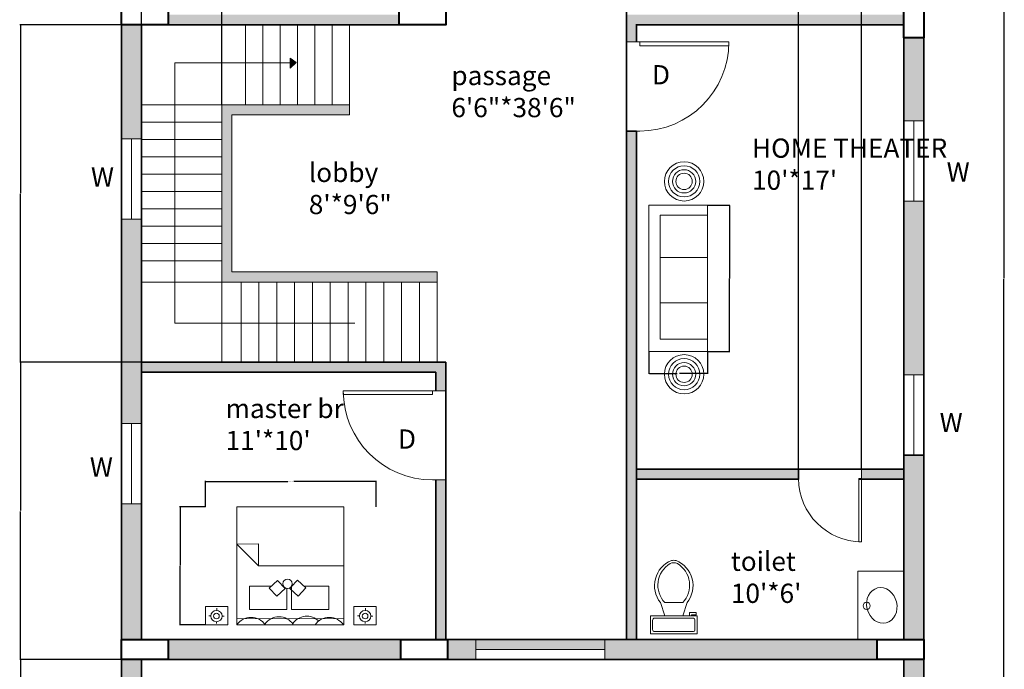
# Model space of a CAD drawing. Units: inches. Extents: x 1568 to 2529, y 2149 to 2897.
# Tile 15 of 16: x 2087 to 2529, y 2326 to 2618. Entities that reach past the tile are written whole.
import ezdxf

# ---------------------------------------------------------------- set-up
doc = ezdxf.new("R2010")
doc.units = ezdxf.units.IN
for name, color, linetype, lineweight in [('A-ANNO-DIMS', 2, 'Continuous', 18), ('A-ANNO-SYMB', 7, 'Continuous', 18), ('A-AREA-IDEN', 210, 'Continuous', 18), ('A-COLS', 7, 'Continuous', 40), ('A-DOOR', 4, 'Continuous', 18), ('A-EQPM', 8, 'Continuous', 18), ('A-FLOR-FIXT', 9, 'Continuous', 18), ('A-FLOR-STRS', 7, 'Continuous', 18), ('A-FURN', 8, 'Continuous', 18), ('A-WALL-PATT', 172, 'Continuous', 13), ('text', 210, 'Continuous', 18), ('wall', 7, 'Continuous', 35), ('window', 130, 'Continuous', 18)]:
    doc.layers.add(name, color=color, linetype=linetype, lineweight=lineweight)
doc.styles.get("Standard").update_dxf_attribs({"font": 'arial.ttf'})
doc.dimstyles.get("Standard").update_dxf_attribs({"dimtxt": 0.18, "dimasz": 0.18, "dimexe": 0.18, "dimexo": 0.0625, "dimgap": 0.09, "dimtad": 0, "dimtih": 1, "dimtoh": 1, "dimdec": 4, "dimzin": 0, "dimdsep": 46, "dimtxsty": 'Standard', "dimcen": 0.09, "dimadec": 0, "dimazin": 0, "dimtfac": 1, "dimtdec": 4, "dimtofl": 0, "dimtmove": 0, "dimatfit": 3, "dimfxl": 1, "dimtolj": 1, "dimtzin": 0, "dimarcsym": 0})

# ---------------------------------------------------------------- blocks, each defined once
blk = doc.blocks.new('*U2')
for p, q in [((0, 0), (0, -6)), ((40, 0), (40, -6))]:
    blk.add_line(p, q)
blk.add_lwpolyline([(0, 0), (0, 40), (1.75, 40), (1.75, 0)], close=True)
blk.add_arc((0, 0), 40, 0, 90)
blk = doc.blocks.new('*U4')
for p, q in [((9.5, -6), (9.5, -2)), ((-10, -8.5), (-8, -8.5)), ((-10, -9.5), (-10, -8.5)), ((-8, -8.5), (-8, -8)), ((-7, -8), (-7, -9.5)), ((-4, -8), (-6, -14)), ((4, -8), (6, -14)), ((-7, -9.5), (-10, -9.5)), ((4, -14), (-4, -14))]:
    blk.add_line(p, q)
blk.add_lwpolyline([(10.5, -8), (10.5, 0), (-10.5, 0), (-10.5, -8)], close=True)
for points in [[(-9.5, -2), (-9.5, -6)], [(8.5, -1), (-8.5, -1)], [(-8.5, -7), (8.5, -7)]]:
    blk.add_lwpolyline(points)
for centre, radius, start, end in [((-8.62, -1.88), 0.884, 81.8699, 188.1301), ((8.62, -1.88), 0.884, 351.8699, 98.1301), ((-8.62, -6.12), 0.884, 171.8699, 278.1301), ((8.62, -6.12), 0.884, 261.8699, 8.1301), ((3.52, -21.58), 12.17, 141.4691, 247.9714), ((4.2, -21.82), 11.33, 136.3677, 238.9468), ((-3.52, -21.58), 12.17, 292.0284, 38.5307), ((-4.2, -21.82), 11.33, 301.053, 43.6321), ((0, -27.88), 4, 245.7318, 294.2682), ((0, -29), 4, 254.8605, 285.1395)]:
    blk.add_arc(centre, radius, start, end)
blk = doc.blocks.new('BED-WITH-NIGHTSTANDS')
for p, q in [((14.05, 36.12), (23.68, 36.4)), ((23.68, 26.45), (14.05, 36.12)), ((23.68, 36.4), (23.68, 26.45)), ((61.95, 26.45), (23.68, 26.45)), ((38.01, 16.14), (37.63, 16.49)), ((38.35, 15.84), (38.01, 16.14)), ((38.35, 16.98), (38.35, 15.84)), ((5, 6.48), (5, 7.42)), ((71.71, 6.48), (71.71, 7.42)), ((2.29, 3.95), (1.38, 3.95)), ((4.92, 1.35), (4.92, 0.55)), ((7.42, 3.92), (8.29, 3.92)), ((14.05, 2.79), (61.95, 2.73)), ((69, 3.95), (68.1, 3.95)), ((71.64, 1.35), (71.64, 0.55)), ((74.13, 3.92), (75, 3.92))]:
    blk.add_line(p, q)
for points in [[(14.05, 0), (61.95, 0), (61.95, 52.9), (14.05, 52.9)], [(31.9, 12.77), (35.7, 16.21), (32.32, 19.94), (28.52, 16.5)], [(10.04, 0), (0, 0), (0, 8.21), (10.04, 8.21)], [(76.49, 0), (66.44, 0), (66.44, 8.21), (76.49, 8.21)]]:
    blk.add_lwpolyline(points, close=True)
for points in [[(38.35, 16.98), (41.16, 20.08), (44.96, 16.64), (41.58, 12.91), (38.01, 16.14)], [(29.36, 17.26), (19.65, 17.26), (19.65, 6.93), (36.45, 6.93), (36.45, 16.34)], [(35.04, 17.26), (34.75, 17.26)], [(38.52, 17.23), (38.52, 6.93), (55.32, 6.93), (55.32, 17.26), (44.28, 17.26)], [(38.6, 17.26), (38.54, 17.26)]]:
    blk.add_lwpolyline(points)
for centre, radius in [((36.79, 18.4), 2.09), ((4.85, 3.92), 2.56), ((4.85, 3.92), 1.27), ((71.57, 3.92), 2.56), ((71.57, 3.92), 1.27)]:
    blk.add_circle(centre, radius)
for centre, start in [((20.4, -4.37), 34.5304), ((32.9, -4.09), 34.5304), ((45.42, -3.86), 46.3255), ((55.47, -4.37), 34.5304)]:
    blk.add_arc(centre, 7.71, start, 145.4696)
blk = doc.blocks.new('SOFA-THREE-SEAT')
for p, q in [((0, 60.18), (0, 65.7)), ((0, 65.7), (26.25, 65.7)), ((26.25, 65.7), (26.25, 0)), ((0, 43.78), (21.18, 43.78)), ((0, 23.43), (21.18, 23.43)), ((0, 0), (0, 5.84)), ((26.25, 0), (0, 0))]:
    blk.add_line(p, q)
blk.add_lwpolyline([(21.18, 60.18), (0, 60.18), (0, 4.48), (21.18, 4.48)], close=True)
blk = doc.blocks.new('TABLE-ROUND-END')
for radius in [8.82, 7, 5.22, 3.67]:
    blk.add_circle((0, 0), radius)
blk = doc.blocks.new('*D17')
at = {"layer": 'A-ANNO-DIMS', "color": 0, "lineweight": -2, "transparency": 16777216}
for p, q in [((2170.58, 2399.15), (2170.58, 2410.74)), ((2170.76, 2410.56), (2207.51, 2410.56)), ((2246.88, 2410.56), (2210.13, 2410.56)), ((2247.06, 2399.15), (2247.06, 2410.74))]:
    blk.add_line(p, q, dxfattribs=at)
at = {"layer": 'A-ANNO-DIMS', "color": 0, "transparency": 16777216}
for points in [[(2170.76, 2410.59), (2170.76, 2410.53), (2170.58, 2410.56)], [(2246.88, 2410.59), (2246.88, 2410.53), (2247.06, 2410.56)]]:
    blk.add_solid(points, dxfattribs=at)
at = {"layer": 'Defpoints', "color": 0, "transparency": 16777216}
for p in [(2247.06, 2410.56), (2170.58, 2399.09), (2247.06, 2399.09)]:
    blk.add_point(p, dxfattribs=at)
at = {"layer": 'A-ANNO-DIMS', "color": 0, "transparency": 16777216, "insert": (2208.82, 2410.56), "char_height": 0.18, "attachment_point": 5}
blk.add_mtext('\\A1;BED GROUP 76 TYP.', dxfattribs=at)
blk = doc.blocks.new('*D18')
at = {"layer": 'A-ANNO-DIMS', "color": 0, "lineweight": -2, "transparency": 16777216}
for p, q in [((2170.51, 2399.09), (2158.92, 2399.09)), ((2159.1, 2398.91), (2159.1, 2372.82)), ((2159.1, 2346.37), (2159.1, 2372.46)), ((2170.51, 2346.19), (2158.92, 2346.19))]:
    blk.add_line(p, q, dxfattribs=at)
at = {"layer": 'A-ANNO-DIMS', "color": 0, "transparency": 16777216}
for points in [[(2159.07, 2398.91), (2159.13, 2398.91), (2159.1, 2399.09)], [(2159.07, 2346.37), (2159.13, 2346.37), (2159.1, 2346.19)]]:
    blk.add_solid(points, dxfattribs=at)
at = {"layer": 'Defpoints', "color": 0, "transparency": 16777216}
for p in [(2159.1, 2399.09), (2170.58, 2399.09), (2170.58, 2346.19)]:
    blk.add_point(p, dxfattribs=at)
at = {"layer": 'A-ANNO-DIMS', "color": 0, "transparency": 16777216, "insert": (2159.1, 2372.64), "char_height": 0.18, "attachment_point": 5}
blk.add_mtext('\\A1;53 TYP.', dxfattribs=at)
blk = doc.blocks.new('*D21')
at = {"layer": 'A-ANNO-DIMS', "color": 0, "lineweight": -2, "transparency": 16777216}
for p, q in [((2395.82, 2534.49), (2405.79, 2534.49)), ((2405.61, 2534.31), (2405.61, 2501.83)), ((2405.61, 2468.98), (2405.61, 2501.46)), ((2395.82, 2468.8), (2405.79, 2468.8))]:
    blk.add_line(p, q, dxfattribs=at)
at = {"layer": 'A-ANNO-DIMS', "color": 0, "transparency": 16777216}
for points in [[(2405.58, 2534.31), (2405.64, 2534.31), (2405.61, 2534.49)], [(2405.58, 2468.98), (2405.64, 2468.98), (2405.61, 2468.8)]]:
    blk.add_solid(points, dxfattribs=at)
at = {"layer": 'Defpoints', "color": 0, "transparency": 16777216}
for p in [(2395.75, 2534.49), (2395.75, 2468.8), (2405.61, 2468.8)]:
    blk.add_point(p, dxfattribs=at)
at = {"layer": 'A-ANNO-DIMS', "color": 0, "transparency": 16777216, "insert": (2405.61, 2501.65), "char_height": 0.18, "attachment_point": 5}
blk.add_mtext('\\A1;SOFA 66 TYP.', dxfattribs=at)
blk = doc.blocks.new('*D22')
at = {"layer": 'A-ANNO-DIMS', "color": 0, "lineweight": -2, "transparency": 16777216}
for p, q in [((2369.51, 2468.74), (2369.51, 2458.76)), ((2395.75, 2468.74), (2395.75, 2458.76)), ((2369.69, 2458.94), (2382.1, 2458.94)), ((2395.57, 2458.94), (2383.16, 2458.94))]:
    blk.add_line(p, q, dxfattribs=at)
at = {"layer": 'A-ANNO-DIMS', "color": 0, "transparency": 16777216}
for points in [[(2369.69, 2458.97), (2369.69, 2458.91), (2369.51, 2458.94)], [(2395.57, 2458.97), (2395.57, 2458.91), (2395.75, 2458.94)]]:
    blk.add_solid(points, dxfattribs=at)
at = {"layer": 'Defpoints', "color": 0, "transparency": 16777216}
for p in [(2369.51, 2468.8), (2395.75, 2468.8), (2369.51, 2458.94)]:
    blk.add_point(p, dxfattribs=at)
at = {"layer": 'A-ANNO-DIMS', "color": 0, "transparency": 16777216, "insert": (2382.63, 2458.94), "char_height": 0.18, "attachment_point": 5}
blk.add_mtext('\\A1;26 TYP.', dxfattribs=at)
blk = doc.blocks.new('*D38')
at = {"layer": 'A-ANNO-DIMS', "color": 0, "lineweight": -2, "transparency": 16777216}
for p, q in [((2492.94, 2801.53), (2528.91, 2801.53)), ((2528.73, 2801.35), (2528.73, 2501.71)), ((2528.73, 2201.71), (2528.73, 2501.35)), ((2492.91, 2201.53), (2528.91, 2201.53))]:
    blk.add_line(p, q, dxfattribs=at)
at = {"layer": 'A-ANNO-DIMS', "color": 0, "transparency": 16777216}
for points in [[(2528.7, 2801.35), (2528.76, 2801.35), (2528.73, 2801.53)], [(2528.7, 2201.71), (2528.76, 2201.71), (2528.73, 2201.53)]]:
    blk.add_solid(points, dxfattribs=at)
at = {"layer": 'Defpoints', "color": 0, "transparency": 16777216}
for p in [(2492.88, 2801.53), (2528.73, 2801.53), (2492.85, 2201.53)]:
    blk.add_point(p, dxfattribs=at)
at = {"layer": 'A-ANNO-DIMS', "color": 0, "transparency": 16777216, "insert": (2528.73, 2501.53), "char_height": 0.18, "attachment_point": 5}
blk.add_mtext('\\A1;600', dxfattribs=at)
blk = doc.blocks.new('*D39')
at = {"layer": 'A-ANNO-DIMS', "color": 0, "lineweight": -2, "transparency": 16777216}
for p, q in [((2132.79, 2330.53), (2087.29, 2330.53)), ((2087.47, 2330.35), (2087.47, 2266.21)), ((2087.47, 2201.71), (2087.47, 2265.85)), ((2132.79, 2201.53), (2087.29, 2201.53))]:
    blk.add_line(p, q, dxfattribs=at)
at = {"layer": 'A-ANNO-DIMS', "color": 0, "transparency": 16777216}
for points in [[(2087.44, 2330.35), (2087.5, 2330.35), (2087.47, 2330.53)], [(2087.44, 2201.71), (2087.5, 2201.71), (2087.47, 2201.53)]]:
    blk.add_solid(points, dxfattribs=at)
at = {"layer": 'Defpoints', "color": 0, "transparency": 16777216}
for p in [(2087.47, 2330.53), (2132.85, 2330.53), (2132.85, 2201.53)]:
    blk.add_point(p, dxfattribs=at)
at = {"layer": 'A-ANNO-DIMS', "color": 0, "transparency": 16777216, "insert": (2087.47, 2266.03), "char_height": 0.18, "attachment_point": 5}
blk.add_mtext('\\A1;129', dxfattribs=at)
blk = doc.blocks.new('*D40')
at = {"layer": 'A-ANNO-DIMS', "color": 0, "lineweight": -2, "transparency": 16777216}
for p, q in [((2141.79, 2464.03), (2087.29, 2464.03)), ((2087.47, 2463.85), (2087.47, 2397.46)), ((2087.47, 2330.71), (2087.47, 2397.1)), ((2141.79, 2330.53), (2087.29, 2330.53))]:
    blk.add_line(p, q, dxfattribs=at)
at = {"layer": 'A-ANNO-DIMS', "color": 0, "transparency": 16777216}
for points in [[(2087.44, 2463.85), (2087.5, 2463.85), (2087.47, 2464.03)], [(2087.44, 2330.71), (2087.5, 2330.71), (2087.47, 2330.53)]]:
    blk.add_solid(points, dxfattribs=at)
at = {"layer": 'Defpoints', "color": 0, "transparency": 16777216}
for p in [(2087.47, 2464.03), (2141.85, 2464.03), (2141.85, 2330.53)]:
    blk.add_point(p, dxfattribs=at)
at = {"layer": 'A-ANNO-DIMS', "color": 0, "transparency": 16777216, "insert": (2087.47, 2397.28), "char_height": 0.18, "attachment_point": 5}
blk.add_mtext('\\A1;133.5', dxfattribs=at)
blk = doc.blocks.new('*D41')
at = {"layer": 'A-ANNO-DIMS', "color": 0, "lineweight": -2, "transparency": 16777216}
for p, q in [((2141.79, 2615.53), (2087.29, 2615.53)), ((2087.47, 2615.35), (2087.47, 2539.96)), ((2087.47, 2464.21), (2087.47, 2539.6)), ((2141.79, 2464.03), (2087.29, 2464.03))]:
    blk.add_line(p, q, dxfattribs=at)
at = {"layer": 'A-ANNO-DIMS', "color": 0, "transparency": 16777216}
for points in [[(2087.44, 2615.35), (2087.5, 2615.35), (2087.47, 2615.53)], [(2087.44, 2464.21), (2087.5, 2464.21), (2087.47, 2464.03)]]:
    blk.add_solid(points, dxfattribs=at)
at = {"layer": 'Defpoints', "color": 0, "transparency": 16777216}
for p in [(2087.47, 2615.53), (2141.85, 2615.53), (2141.85, 2464.03)]:
    blk.add_point(p, dxfattribs=at)
at = {"layer": 'A-ANNO-DIMS', "color": 0, "transparency": 16777216, "insert": (2087.47, 2539.78), "char_height": 0.18, "attachment_point": 5}
blk.add_mtext('\\A1;151.5', dxfattribs=at)
blk = doc.blocks.new('*D42')
at = {"layer": 'A-ANNO-DIMS', "color": 0, "lineweight": -2, "transparency": 16777216}
for p, q in [((2141.85, 2579.59), (2141.85, 2896.84)), ((2142.03, 2896.66), (2159.63, 2896.66)), ((2177.67, 2896.66), (2160.07, 2896.66)), ((2177.85, 2579.59), (2177.85, 2896.84))]:
    blk.add_line(p, q, dxfattribs=at)
at = {"layer": 'A-ANNO-DIMS', "color": 0, "transparency": 16777216}
for points in [[(2142.03, 2896.69), (2142.03, 2896.63), (2141.85, 2896.66)], [(2177.67, 2896.69), (2177.67, 2896.63), (2177.85, 2896.66)]]:
    blk.add_solid(points, dxfattribs=at)
at = {"layer": 'Defpoints', "color": 0, "transparency": 16777216}
for p in [(2177.85, 2896.66), (2141.85, 2579.53), (2177.85, 2579.53)]:
    blk.add_point(p, dxfattribs=at)
at = {"layer": 'A-ANNO-DIMS', "color": 0, "transparency": 16777216, "insert": (2159.85, 2896.66), "char_height": 0.18, "attachment_point": 5}
blk.add_mtext('\\A1;36', dxfattribs=at)
blk = doc.blocks.new('*D45')
at = {"layer": 'A-ANNO-DIMS', "color": 0, "lineweight": -2, "transparency": 16777216}
for p, q in [((2436.62, 2416.09), (2436.62, 2896.84)), ((2436.8, 2896.66), (2450.31, 2896.66)), ((2464.75, 2896.66), (2451.24, 2896.66)), ((2464.93, 2416.09), (2464.93, 2896.84))]:
    blk.add_line(p, q, dxfattribs=at)
at = {"layer": 'A-ANNO-DIMS', "color": 0, "transparency": 16777216}
for points in [[(2436.8, 2896.69), (2436.8, 2896.63), (2436.62, 2896.66)], [(2464.75, 2896.69), (2464.75, 2896.63), (2464.93, 2896.66)]]:
    blk.add_solid(points, dxfattribs=at)
at = {"layer": 'Defpoints', "color": 0, "transparency": 16777216}
for p in [(2464.93, 2896.66), (2436.62, 2416.03), (2464.93, 2416.03)]:
    blk.add_point(p, dxfattribs=at)
at = {"layer": 'A-ANNO-DIMS', "color": 0, "transparency": 16777216, "insert": (2450.77, 2896.66), "char_height": 0.18, "attachment_point": 5}
blk.add_mtext('\\A1;28.305', dxfattribs=at)

msp = doc.modelspace()

# ---------------------------------------------------------------- hatches: boundary and pattern name
at = {"layer": 'A-ANNO-SYMB'}
h = msp.add_hatch(color=256, dxfattribs=at)
h.dxf.hatch_style = 1
h.paths.add_polyline_path([(2211.1402, 2598.4963), (2208.5798, 2600.5832), (2208.5798, 2596.9578), (2208.5798, 2595.9578)])
at = {"layer": 'A-WALL-PATT'}
h = msp.add_hatch(color=256, dxfattribs=at)
h.dxf.hatch_style = 1
h.paths.add_polyline_path([(2257.4593, 2801.532), (2153.7841, 2801.532), (2153.7841, 2792.532), (2257.4593, 2792.532)])
h.paths.add_polyline_path([(2331.7115, 2801.532), (2278.3925, 2801.532), (2278.3925, 2792.532), (2331.7115, 2792.532)])
h.paths.add_polyline_path([(2141.8509, 2753.3576), (2141.6865, 2753.3576), (2132.8509, 2753.3576), (2132.8509, 2705.9172), (2141.8509, 2705.9172)])
h.paths.add_polyline_path([(2278.3509, 2757.9833), (2274.1052, 2757.9833, -0.00224577), (2273.8509, 2757.9844), (2273.8509, 2744.532), (2141.8509, 2744.532), (2141.8509, 2740.032), (2273.8509, 2740.032), (2273.8509, 2730.8156), (2278.3509, 2730.8156), (2278.3509, 2740.032)])
h.paths.add_polyline_path([(2471.947, 2801.532), (2367.7115, 2801.532), (2367.7115, 2792.532), (2471.947, 2792.532)])
h.paths.add_polyline_path([(2402.7886, 2351.2573), (2436.5067, 2351.2573), (2436.5067, 2383.453), (2402.7886, 2383.453)], flags=9)
h.paths.add_polyline_path([(2363.115, 2703.2844), (2384.1733, 2703.2844), (2384.1733, 2721.0645), (2363.115, 2721.0645)], flags=9)
h.paths.add_polyline_path([(2367.7631, 2584.032), (2380.7818, 2584.032), (2380.7818, 2601.8121), (2367.7631, 2601.8121)], flags=9)
h.paths.add_polyline_path([(2412.2706, 2522.1491), (2473.8683, 2522.1491), (2473.8683, 2568.725), (2412.2706, 2568.725)], flags=9)
h.paths.add_polyline_path([(2412.2706, 2686.5293), (2474.6569, 2686.5293), (2474.6569, 2718.725), (2412.2706, 2718.725)], flags=9)
h.paths.add_polyline_path([(2305.8704, 2205.7429), (2329.6007, 2205.7429), (2329.6007, 2223.523), (2305.8704, 2223.523)], flags=9)
h.paths.add_polyline_path([(2312.4696, 2308.5242), (2328.1604, 2308.5242), (2328.1604, 2326.3043), (2312.4696, 2326.3043)], flags=9)
h.paths.add_polyline_path([(2253.7912, 2420.5203), (2266.8099, 2420.5203), (2266.8099, 2438.3004), (2253.7912, 2438.3004)], flags=9)
h.paths.add_polyline_path([(2261.5714, 2703.4315), (2274.5902, 2703.4315), (2274.5902, 2721.2116), (2261.5714, 2721.2116)], flags=9)
h.paths.add_polyline_path([(2277.898, 2569.2764), (2333.9221, 2569.2764), (2333.9221, 2601.4721), (2277.898, 2601.4721)], flags=9)
h.paths.add_polyline_path([(2176.0749, 2419.8331), (2231.9754, 2419.8331), (2231.9754, 2452.0288), (2176.0749, 2452.0288)], flags=9)
h.paths.add_polyline_path([(2213.9423, 2525.7697), (2252.2216, 2525.7697), (2252.2216, 2557.9653), (2213.9423, 2557.9653)], flags=9)
h.paths.add_polyline_path([(2170.6878, 2692.4783), (2211.1801, 2692.4783), (2211.1801, 2724.6739), (2170.6878, 2724.6739)], flags=9)
h.paths.add_polyline_path([(2262.4629, 2764.5694), (2275.4816, 2764.5694), (2275.4816, 2782.3495), (2262.4629, 2782.3495)], flags=9)
h.paths.add_polyline_path([(2183.6493, 2749.7187), (2217.3673, 2749.7187), (2217.3673, 2781.9143), (2183.6493, 2781.9143)], flags=9)
h = msp.add_hatch(color=256, dxfattribs=at)
h.dxf.hatch_style = 1
h.paths.add_polyline_path([(2492.8509, 2792.532), (2483.8509, 2792.532), (2483.8509, 2699.1671), (2492.8509, 2699.1671)])
h.paths.add_polyline_path([(2278.3509, 2690.8156), (2273.8509, 2690.8156), (2273.8509, 2624.532), (2278.3509, 2624.532)])
h.paths.add_polyline_path([(2257.4177, 2620.032), (2153.7841, 2620.032), (2153.7841, 2615.532), (2257.4177, 2615.532)])
h.paths.add_polyline_path([(2141.8509, 2669.9172), (2132.8509, 2669.9172), (2132.8509, 2624.532), (2141.8509, 2624.532)])
h.paths.add_polyline_path([(2402.7886, 2351.2573), (2436.5067, 2351.2573), (2436.5067, 2383.453), (2402.7886, 2383.453)], flags=9)
h.paths.add_polyline_path([(2363.115, 2703.2844), (2384.1733, 2703.2844), (2384.1733, 2721.0645), (2363.115, 2721.0645)], flags=9)
h.paths.add_polyline_path([(2367.7631, 2584.032), (2380.7818, 2584.032), (2380.7818, 2601.8121), (2367.7631, 2601.8121)], flags=9)
h.paths.add_polyline_path([(2412.2706, 2522.1491), (2473.8683, 2522.1491), (2473.8683, 2568.725), (2412.2706, 2568.725)], flags=9)
h.paths.add_polyline_path([(2412.2706, 2686.5293), (2474.6569, 2686.5293), (2474.6569, 2718.725), (2412.2706, 2718.725)], flags=9)
h.paths.add_polyline_path([(2305.8704, 2205.7429), (2329.6007, 2205.7429), (2329.6007, 2223.523), (2305.8704, 2223.523)], flags=9)
h.paths.add_polyline_path([(2312.4696, 2308.5242), (2328.1604, 2308.5242), (2328.1604, 2326.3043), (2312.4696, 2326.3043)], flags=9)
h.paths.add_polyline_path([(2253.7912, 2420.5203), (2266.8099, 2420.5203), (2266.8099, 2438.3004), (2253.7912, 2438.3004)], flags=9)
h.paths.add_polyline_path([(2261.5714, 2703.4315), (2274.5902, 2703.4315), (2274.5902, 2721.2116), (2261.5714, 2721.2116)], flags=9)
h.paths.add_polyline_path([(2262.4629, 2764.5694), (2275.4816, 2764.5694), (2275.4816, 2782.3495), (2262.4629, 2782.3495)], flags=9)
h.paths.add_polyline_path([(2277.898, 2569.2764), (2333.9221, 2569.2764), (2333.9221, 2601.4721), (2277.898, 2601.4721)], flags=9)
h.paths.add_polyline_path([(2176.0749, 2419.8331), (2231.9754, 2419.8331), (2231.9754, 2452.0288), (2176.0749, 2452.0288)], flags=9)
h.paths.add_polyline_path([(2213.9423, 2525.7697), (2252.2216, 2525.7697), (2252.2216, 2557.9653), (2213.9423, 2557.9653)], flags=9)
h.paths.add_polyline_path([(2170.6878, 2692.4783), (2211.1801, 2692.4783), (2211.1801, 2724.6739), (2170.6878, 2724.6739)], flags=9)
h.paths.add_polyline_path([(2183.6493, 2749.7187), (2217.3673, 2749.7187), (2217.3673, 2781.9143), (2183.6493, 2781.9143)], flags=9)
h = msp.add_hatch(color=256, dxfattribs=at)
h.dxf.hatch_style = 1
h.paths.add_polyline_path([(2141.8509, 2615.532), (2132.8509, 2615.532), (2132.8509, 2564.2764), (2141.8509, 2564.2764)])
h.paths.add_polyline_path([(2141.8509, 2528.2764), (2132.8509, 2528.2764), (2132.8509, 2436.512), (2141.8509, 2436.512), (2141.8509, 2459.532)])
h.paths.add_polyline_path([(2278.3509, 2464.032), (2253.6925, 2464.032), (2141.8509, 2464.032), (2141.8509, 2459.532), (2255.8509, 2459.532), (2273.8509, 2459.532), (2273.8509, 2451.2271), (2278.3509, 2451.2271)])
h.paths.add_polyline_path([(2141.8509, 2400.512), (2132.8509, 2400.512), (2132.8509, 2339.532), (2141.8509, 2339.532)])
h.paths.add_polyline_path([(2258.2144, 2339.532), (2153.7841, 2339.532), (2153.7841, 2330.532), (2258.2144, 2330.532)])
h.paths.add_polyline_path([(2291.8353, 2339.532), (2279.1476, 2339.532), (2279.1476, 2330.532), (2291.8353, 2330.532)])
h.paths.add_polyline_path([(2402.7886, 2351.2573), (2436.5067, 2351.2573), (2436.5067, 2383.453), (2402.7886, 2383.453)], flags=9)
h.paths.add_polyline_path([(2363.115, 2703.2844), (2384.1733, 2703.2844), (2384.1733, 2721.0645), (2363.115, 2721.0645)], flags=9)
h.paths.add_polyline_path([(2367.7631, 2584.032), (2380.7818, 2584.032), (2380.7818, 2601.8121), (2367.7631, 2601.8121)], flags=9)
h.paths.add_polyline_path([(2412.2706, 2522.1491), (2473.8683, 2522.1491), (2473.8683, 2568.725), (2412.2706, 2568.725)], flags=9)
h.paths.add_polyline_path([(2412.2706, 2686.5293), (2474.6569, 2686.5293), (2474.6569, 2718.725), (2412.2706, 2718.725)], flags=9)
h.paths.add_polyline_path([(2305.8704, 2205.7429), (2329.6007, 2205.7429), (2329.6007, 2223.523), (2305.8704, 2223.523)], flags=9)
h.paths.add_polyline_path([(2312.4696, 2308.5242), (2328.1604, 2308.5242), (2328.1604, 2326.3043), (2312.4696, 2326.3043)], flags=9)
h.paths.add_polyline_path([(2261.5714, 2703.4315), (2274.5902, 2703.4315), (2274.5902, 2721.2116), (2261.5714, 2721.2116)], flags=9)
h.paths.add_polyline_path([(2262.4629, 2764.5694), (2275.4816, 2764.5694), (2275.4816, 2782.3495), (2262.4629, 2782.3495)], flags=9)
h.paths.add_polyline_path([(2277.898, 2569.2764), (2333.9221, 2569.2764), (2333.9221, 2601.4721), (2277.898, 2601.4721)], flags=9)
h.paths.add_polyline_path([(2213.9423, 2525.7697), (2252.2216, 2525.7697), (2252.2216, 2557.9653), (2213.9423, 2557.9653)], flags=9)
h.paths.add_polyline_path([(2170.6878, 2692.4783), (2211.1801, 2692.4783), (2211.1801, 2724.6739), (2170.6878, 2724.6739)], flags=9)
h.paths.add_polyline_path([(2183.6493, 2749.7187), (2217.3673, 2749.7187), (2217.3673, 2781.9143), (2183.6493, 2781.9143)], flags=9)
h = msp.add_hatch(color=256, dxfattribs=at)
h.dxf.hatch_style = 1
h.paths.add_polyline_path([(2492.8509, 2663.1671), (2483.8509, 2663.1671), (2483.8509, 2630.5978), (2492.8509, 2630.5978)])
h.paths.add_polyline_path([(2492.8509, 2609.6646), (2483.8509, 2609.6646), (2483.8509, 2572.3679), (2492.8509, 2572.3679)])
h.paths.add_polyline_path([(2492.8509, 2536.3679), (2483.8509, 2536.3679), (2483.8509, 2476.032), (2483.8509, 2458.371), (2492.8509, 2458.371)])
h.paths.add_polyline_path([(2483.8509, 2620.032), (2361.425, 2620.032), (2359.3509, 2620.032), (2359.3509, 2607.8035), (2363.8509, 2607.8035), (2363.8509, 2615.532), (2483.8509, 2615.532)])
h.paths.add_polyline_path([(2402.7886, 2351.2573), (2436.5067, 2351.2573), (2436.5067, 2383.453), (2402.7886, 2383.453)], flags=9)
h.paths.add_polyline_path([(2412.2706, 2522.1491), (2473.8683, 2522.1491), (2473.8683, 2568.725), (2412.2706, 2568.725)], flags=9)
h.paths.add_polyline_path([(2305.8704, 2205.7429), (2329.6007, 2205.7429), (2329.6007, 2223.523), (2305.8704, 2223.523)], flags=9)
h.paths.add_polyline_path([(2312.4696, 2308.5242), (2328.1604, 2308.5242), (2328.1604, 2326.3043), (2312.4696, 2326.3043)], flags=9)
h.paths.add_polyline_path([(2253.7912, 2420.5203), (2266.8099, 2420.5203), (2266.8099, 2438.3004), (2253.7912, 2438.3004)], flags=9)
h.paths.add_polyline_path([(2261.5714, 2703.4315), (2274.5902, 2703.4315), (2274.5902, 2721.2116), (2261.5714, 2721.2116)], flags=9)
h.paths.add_polyline_path([(2262.4629, 2764.5694), (2275.4816, 2764.5694), (2275.4816, 2782.3495), (2262.4629, 2782.3495)], flags=9)
h.paths.add_polyline_path([(2277.898, 2569.2764), (2333.9221, 2569.2764), (2333.9221, 2601.4721), (2277.898, 2601.4721)], flags=9)
h.paths.add_polyline_path([(2176.0749, 2419.8331), (2231.9754, 2419.8331), (2231.9754, 2452.0288), (2176.0749, 2452.0288)], flags=9)
h.paths.add_polyline_path([(2213.9423, 2525.7697), (2252.2216, 2525.7697), (2252.2216, 2557.9653), (2213.9423, 2557.9653)], flags=9)
h.paths.add_polyline_path([(2170.6878, 2692.4783), (2211.1801, 2692.4783), (2211.1801, 2724.6739), (2170.6878, 2724.6739)], flags=9)
h.paths.add_polyline_path([(2183.6493, 2749.7187), (2217.3673, 2749.7187), (2217.3673, 2781.9143), (2183.6493, 2781.9143)], flags=9)
h = msp.add_hatch(color=256, dxfattribs=at)
h.dxf.hatch_style = 1
h.paths.add_polyline_path([(2471.9177, 2339.532), (2463.2103, 2339.532), (2350.013, 2339.532), (2311.8757, 2339.532), (2291.8353, 2339.532), (2291.8353, 2335.032), (2313.7499, 2335.032), (2349.7476, 2335.032), (2349.7476, 2330.532), (2471.9177, 2330.532)])
h.paths.add_polyline_path([(2363.115, 2703.2844), (2384.1733, 2703.2844), (2384.1733, 2721.0645), (2363.115, 2721.0645)], flags=9)
h.paths.add_polyline_path([(2367.7631, 2584.032), (2380.7818, 2584.032), (2380.7818, 2601.8121), (2367.7631, 2601.8121)], flags=9)
h.paths.add_polyline_path([(2412.2706, 2522.1491), (2473.8683, 2522.1491), (2473.8683, 2568.725), (2412.2706, 2568.725)], flags=9)
h.paths.add_polyline_path([(2412.2706, 2686.5293), (2474.6569, 2686.5293), (2474.6569, 2718.725), (2412.2706, 2718.725)], flags=9)
h.paths.add_polyline_path([(2253.7912, 2420.5203), (2266.8099, 2420.5203), (2266.8099, 2438.3004), (2253.7912, 2438.3004)], flags=9)
h.paths.add_polyline_path([(2261.5714, 2703.4315), (2274.5902, 2703.4315), (2274.5902, 2721.2116), (2261.5714, 2721.2116)], flags=9)
h.paths.add_polyline_path([(2262.4629, 2764.5694), (2275.4816, 2764.5694), (2275.4816, 2782.3495), (2262.4629, 2782.3495)], flags=9)
h.paths.add_polyline_path([(2277.898, 2569.2764), (2333.9221, 2569.2764), (2333.9221, 2601.4721), (2277.898, 2601.4721)], flags=9)
h.paths.add_polyline_path([(2176.0749, 2419.8331), (2231.9754, 2419.8331), (2231.9754, 2452.0288), (2176.0749, 2452.0288)], flags=9)
h.paths.add_polyline_path([(2213.9423, 2525.7697), (2252.2216, 2525.7697), (2252.2216, 2557.9653), (2213.9423, 2557.9653)], flags=9)
h.paths.add_polyline_path([(2170.6878, 2692.4783), (2211.1801, 2692.4783), (2211.1801, 2724.6739), (2170.6878, 2724.6739)], flags=9)
h.paths.add_polyline_path([(2183.6493, 2749.7187), (2217.3673, 2749.7187), (2217.3673, 2781.9143), (2183.6493, 2781.9143)], flags=9)
h = msp.add_hatch(color=256, dxfattribs=at)
h.dxf.hatch_style = 1
h.paths.add_polyline_path([(2492.8509, 2422.371), (2483.8509, 2422.371), (2483.8509, 2339.532), (2492.8509, 2339.532)])
h.paths.add_polyline_path([(2483.8509, 2416.032), (2464.9258, 2416.032), (2464.9258, 2411.7863), (2464.9258, 2411.532), (2483.8509, 2411.532)])
h.paths.add_polyline_path([(2402.7886, 2351.2573), (2436.5067, 2351.2573), (2436.5067, 2383.453), (2402.7886, 2383.453)], flags=9)
h.paths.add_polyline_path([(2363.115, 2703.2844), (2384.1733, 2703.2844), (2384.1733, 2721.0645), (2363.115, 2721.0645)], flags=9)
h.paths.add_polyline_path([(2367.7631, 2584.032), (2380.7818, 2584.032), (2380.7818, 2601.8121), (2367.7631, 2601.8121)], flags=9)
h.paths.add_polyline_path([(2412.2706, 2522.1491), (2473.8683, 2522.1491), (2473.8683, 2568.725), (2412.2706, 2568.725)], flags=9)
h.paths.add_polyline_path([(2412.2706, 2686.5293), (2474.6569, 2686.5293), (2474.6569, 2718.725), (2412.2706, 2718.725)], flags=9)
h.paths.add_polyline_path([(2305.8704, 2205.7429), (2329.6007, 2205.7429), (2329.6007, 2223.523), (2305.8704, 2223.523)], flags=9)
h.paths.add_polyline_path([(2312.4696, 2308.5242), (2328.1604, 2308.5242), (2328.1604, 2326.3043), (2312.4696, 2326.3043)], flags=9)
h.paths.add_polyline_path([(2253.7912, 2420.5203), (2266.8099, 2420.5203), (2266.8099, 2438.3004), (2253.7912, 2438.3004)], flags=9)
h.paths.add_polyline_path([(2261.5714, 2703.4315), (2274.5902, 2703.4315), (2274.5902, 2721.2116), (2261.5714, 2721.2116)], flags=9)
h.paths.add_polyline_path([(2262.4629, 2764.5694), (2275.4816, 2764.5694), (2275.4816, 2782.3495), (2262.4629, 2782.3495)], flags=9)
h.paths.add_polyline_path([(2277.898, 2569.2764), (2333.9221, 2569.2764), (2333.9221, 2601.4721), (2277.898, 2601.4721)], flags=9)
h.paths.add_polyline_path([(2176.0749, 2419.8331), (2231.9754, 2419.8331), (2231.9754, 2452.0288), (2176.0749, 2452.0288)], flags=9)
h.paths.add_polyline_path([(2213.9423, 2525.7697), (2252.2216, 2525.7697), (2252.2216, 2557.9653), (2213.9423, 2557.9653)], flags=9)
h.paths.add_polyline_path([(2170.6878, 2692.4783), (2211.1801, 2692.4783), (2211.1801, 2724.6739), (2170.6878, 2724.6739)], flags=9)
h.paths.add_polyline_path([(2183.6493, 2749.7187), (2217.3673, 2749.7187), (2217.3673, 2781.9143), (2183.6493, 2781.9143)], flags=9)
h = msp.add_hatch(color=256, dxfattribs=at)
h.dxf.hatch_style = 1
h.paths.add_polyline_path([(2436.6209, 2416.032), (2363.8509, 2416.032), (2363.8509, 2411.532), (2436.6209, 2411.532)])
h.paths.add_polyline_path([(2363.115, 2703.2844), (2384.1733, 2703.2844), (2384.1733, 2721.0645), (2363.115, 2721.0645)], flags=9)
h.paths.add_polyline_path([(2367.7631, 2584.032), (2380.7818, 2584.032), (2380.7818, 2601.8121), (2367.7631, 2601.8121)], flags=9)
h.paths.add_polyline_path([(2412.2706, 2522.1491), (2473.8683, 2522.1491), (2473.8683, 2568.725), (2412.2706, 2568.725)], flags=9)
h.paths.add_polyline_path([(2412.2706, 2686.5293), (2474.6569, 2686.5293), (2474.6569, 2718.725), (2412.2706, 2718.725)], flags=9)
h.paths.add_polyline_path([(2261.5714, 2703.4315), (2274.5902, 2703.4315), (2274.5902, 2721.2116), (2261.5714, 2721.2116)], flags=9)
h.paths.add_polyline_path([(2262.4629, 2764.5694), (2275.4816, 2764.5694), (2275.4816, 2782.3495), (2262.4629, 2782.3495)], flags=9)
h.paths.add_polyline_path([(2277.898, 2569.2764), (2333.9221, 2569.2764), (2333.9221, 2601.4721), (2277.898, 2601.4721)], flags=9)
h.paths.add_polyline_path([(2213.9423, 2525.7697), (2252.2216, 2525.7697), (2252.2216, 2557.9653), (2213.9423, 2557.9653)], flags=9)
h.paths.add_polyline_path([(2170.6878, 2692.4783), (2211.1801, 2692.4783), (2211.1801, 2724.6739), (2170.6878, 2724.6739)], flags=9)
h.paths.add_polyline_path([(2183.6493, 2749.7187), (2217.3673, 2749.7187), (2217.3673, 2781.9143), (2183.6493, 2781.9143)], flags=9)
h.paths.add_polyline_path([(2402.7886, 2351.2573), (2436.5067, 2351.2573), (2436.5067, 2383.453), (2402.7886, 2383.453)], flags=9)
h.paths.add_polyline_path([(2305.8704, 2205.7429), (2329.6007, 2205.7429), (2329.6007, 2223.523), (2305.8704, 2223.523)], flags=9)
h.paths.add_polyline_path([(2312.4696, 2308.5242), (2328.1604, 2308.5242), (2328.1604, 2326.3043), (2312.4696, 2326.3043)], flags=9)
h.paths.add_polyline_path([(2253.7912, 2420.5203), (2266.8099, 2420.5203), (2266.8099, 2438.3004), (2253.7912, 2438.3004)], flags=9)
h.paths.add_polyline_path([(2176.0749, 2419.8331), (2231.9754, 2419.8331), (2231.9754, 2452.0288), (2176.0749, 2452.0288)], flags=9)
h = msp.add_hatch(color=256, dxfattribs=at)
h.dxf.hatch_style = 1
h.paths.add_polyline_path([(2278.3509, 2411.2271), (2273.8509, 2411.2271), (2273.8509, 2339.532), (2278.3509, 2339.532)])
h.paths.add_polyline_path([(2363.115, 2703.2844), (2384.1733, 2703.2844), (2384.1733, 2721.0645), (2363.115, 2721.0645)], flags=9)
h.paths.add_polyline_path([(2367.7631, 2584.032), (2380.7818, 2584.032), (2380.7818, 2601.8121), (2367.7631, 2601.8121)], flags=9)
h.paths.add_polyline_path([(2412.2706, 2522.1491), (2473.8683, 2522.1491), (2473.8683, 2568.725), (2412.2706, 2568.725)], flags=9)
h.paths.add_polyline_path([(2412.2706, 2686.5293), (2474.6569, 2686.5293), (2474.6569, 2718.725), (2412.2706, 2718.725)], flags=9)
h.paths.add_polyline_path([(2261.5714, 2703.4315), (2274.5902, 2703.4315), (2274.5902, 2721.2116), (2261.5714, 2721.2116)], flags=9)
h.paths.add_polyline_path([(2262.4629, 2764.5694), (2275.4816, 2764.5694), (2275.4816, 2782.3495), (2262.4629, 2782.3495)], flags=9)
h.paths.add_polyline_path([(2277.898, 2569.2764), (2333.9221, 2569.2764), (2333.9221, 2601.4721), (2277.898, 2601.4721)], flags=9)
h.paths.add_polyline_path([(2213.9423, 2525.7697), (2252.2216, 2525.7697), (2252.2216, 2557.9653), (2213.9423, 2557.9653)], flags=9)
h.paths.add_polyline_path([(2170.6878, 2692.4783), (2211.1801, 2692.4783), (2211.1801, 2724.6739), (2170.6878, 2724.6739)], flags=9)
h.paths.add_polyline_path([(2183.6493, 2749.7187), (2217.3673, 2749.7187), (2217.3673, 2781.9143), (2183.6493, 2781.9143)], flags=9)
h = msp.add_hatch(color=256, dxfattribs=at)
h.dxf.hatch_style = 1
h.paths.add_polyline_path([(2235.0675, 2579.532), (2177.8509, 2579.532), (2177.8509, 2500.032), (2274.4826, 2500.032), (2274.4826, 2504.532), (2182.3509, 2504.532), (2182.3509, 2575.032), (2235.0675, 2575.032)])
h = msp.add_hatch(color=256, dxfattribs=at)
h.dxf.hatch_style = 1
h.paths.add_polyline_path([(2363.8509, 2567.8035), (2359.3509, 2567.8035), (2359.3509, 2339.532), (2363.8509, 2339.532)])
h = msp.add_hatch(color=256, dxfattribs=at)
h.dxf.hatch_style = 1
h.paths.add_polyline_path([(2492.8509, 2330.532), (2483.8509, 2330.532), (2483.8509, 2210.532), (2367.8146, 2210.532), (2367.8146, 2201.532), (2492.8509, 2201.532)])
h.paths.add_polyline_path([(2141.8509, 2330.532), (2132.8509, 2330.532), (2132.8509, 2201.532), (2271.818, 2201.532), (2271.818, 2210.532), (2141.8509, 2210.532)])

# ---------------------------------------------------------------- linework, layer by layer
at = {"layer": 'A-ANNO-SYMB'}
for p, q in [((2156.8103, 2481.5328), (2156.8103, 2598.3459)), ((2156.8103, 2598.3459), (2208.5798, 2598.3459)), ((2208.5798, 2598.3459), (2208.5798, 2600.5832)), ((2208.5798, 2600.5832), (2208.5798, 2596.9578)), ((2211.1402, 2598.4963), (2208.5798, 2600.5832)), ((2208.5798, 2595.9578), (2211.1402, 2598.4963)), ((2208.5798, 2596.9578), (2208.5798, 2595.9578)), ((2237.5027, 2481.5328), (2156.8103, 2481.5328))]:
    msp.add_line(p, q, dxfattribs=at)
at = {"layer": 'A-COLS'}
for points in [[(2492.8509, 2630.5978), (2492.8509, 2609.6646), (2483.8509, 2609.6646), (2483.8509, 2630.5978)], [(2132.8509, 2624.532), (2153.7841, 2624.532), (2153.7841, 2615.532), (2132.8509, 2615.532)], [(2257.4177, 2624.532), (2278.3509, 2624.532), (2278.3509, 2615.532), (2257.4177, 2615.532)], [(2132.8509, 2339.532), (2153.7841, 2339.532), (2153.7841, 2330.532), (2132.8509, 2330.532)], [(2258.2144, 2339.532), (2279.1476, 2339.532), (2279.1476, 2330.532), (2258.2144, 2330.532)], [(2471.9177, 2339.532), (2492.8509, 2339.532), (2492.8509, 2330.532), (2471.9177, 2330.532)]]:
    msp.add_lwpolyline(points, close=True, dxfattribs=at)
at = {"layer": 'A-EQPM'}
msp.add_lwpolyline([(2483.8509, 2476.032), (2483.8509, 2476.032), (2483.8509, 2476.032), (2483.8509, 2476.032)], close=True, dxfattribs=at)
at = {"layer": 'A-FLOR-FIXT'}
msp.add_lwpolyline([(2483.8509, 2339.532), (2463.2103, 2339.532), (2463.2103, 2370.2883), (2483.8509, 2370.2883)], close=True, dxfattribs=at)
msp.add_circle((2467.1763, 2354.6869), 1.61, dxfattribs=at)
msp.add_ellipse((2473.9843, 2354.8496), major_axis=(1.9128, -7.8464), ratio=0.83744645, dxfattribs=at)
at = {"layer": 'A-FLOR-STRS'}
for p, q in [((2177.8509, 2579.532), (2177.8509, 2615.532)), ((2177.8509, 2615.532), (2177.8509, 2464.032)), ((2188.4172, 2615.532), (2188.4172, 2579.532)), ((2196.1922, 2615.532), (2196.1922, 2579.532)), ((2203.9673, 2615.532), (2203.9673, 2579.532)), ((2211.7424, 2615.532), (2211.7424, 2579.532)), ((2219.5174, 2615.532), (2219.5174, 2579.532)), ((2227.2925, 2615.532), (2227.2925, 2579.532)), ((2235.0675, 2615.532), (2235.0675, 2579.532)), ((2235.0675, 2575.032), (2235.0675, 2588.6853)), ((2177.8509, 2579.532), (2141.8509, 2579.532)), ((2177.8509, 2500.032), (2177.8509, 2579.532)), ((2235.0675, 2579.532), (2177.8509, 2579.532)), ((2177.8509, 2571.7569), (2141.8509, 2571.7569)), ((2182.3509, 2504.532), (2182.3509, 2575.032)), ((2235.0675, 2575.032), (2182.3509, 2575.032)), ((2177.8509, 2563.9819), (2141.8509, 2563.9819)), ((2177.8509, 2556.2068), (2141.8509, 2556.2068)), ((2177.8509, 2548.4318), (2141.8509, 2548.4318)), ((2177.8509, 2540.6567), (2141.8509, 2540.6567)), ((2177.8509, 2532.8817), (2141.8509, 2532.8817)), ((2177.8509, 2525.1066), (2141.8509, 2525.1066)), ((2177.8509, 2517.3315), (2141.8509, 2517.3315)), ((2177.8509, 2509.5565), (2141.8509, 2509.5565)), ((2274.4826, 2504.532), (2182.3509, 2504.532)), ((2274.4826, 2504.532), (2274.4826, 2490.3293)), ((2177.8509, 2500.032), (2141.8509, 2500.032)), ((2274.4826, 2500.032), (2177.8509, 2500.032)), ((2186.4826, 2464.032), (2186.4826, 2500.032)), ((2194.4826, 2464.032), (2194.4826, 2500.032)), ((2202.4826, 2464.032), (2202.4826, 2500.032)), ((2210.4826, 2464.032), (2210.4826, 2500.032)), ((2218.4826, 2464.032), (2218.4826, 2500.032)), ((2226.4826, 2464.032), (2226.4826, 2500.032)), ((2234.4826, 2464.032), (2234.4826, 2500.032)), ((2242.4826, 2464.032), (2242.4826, 2500.032)), ((2250.4826, 2464.032), (2250.4826, 2500.032)), ((2258.4826, 2464.032), (2258.4826, 2500.032)), ((2266.4826, 2464.032), (2266.4826, 2500.032)), ((2274.4826, 2464.032), (2274.4826, 2500.032)), ((2141.8509, 2464.032), (2177.8509, 2464.032))]:
    msp.add_line(p, q, dxfattribs=at)
at = {"layer": 'wall'}
for p, q in [((2359.3509, 2600.532), (2359.3509, 2792.532)), ((2483.8509, 2792.532), (2483.8509, 2615.532)), ((2278.3509, 2740.032), (2278.3509, 2615.532)), ((2278.3509, 2615.532), (2141.8509, 2615.532)), ((2141.8509, 2615.532), (2141.8509, 2519.532)), ((2483.8509, 2615.532), (2363.6781, 2615.532)), ((2363.8509, 2607.8035), (2363.8509, 2615.532)), ((2359.3509, 2600.532), (2359.3509, 2476.032)), ((2483.8509, 2476.032), (2483.8509, 2596.032)), ((2363.8509, 2510.0763), (2363.8509, 2567.8035)), ((2363.8509, 2510.0763), (2363.8509, 2476.032)), ((2363.8509, 2460.3505), (2363.8509, 2496.3094)), ((2359.3509, 2339.532), (2359.3509, 2476.032)), ((2363.8509, 2339.532), (2363.8509, 2471.532)), ((2141.8509, 2464.032), (2255.8509, 2464.032)), ((2278.3509, 2464.032), (2253.6925, 2464.032)), ((2278.3509, 2339.532), (2278.3509, 2464.032)), ((2141.8509, 2459.532), (2255.8509, 2459.532)), ((2141.8509, 2459.532), (2141.8509, 2339.532)), ((2273.8509, 2459.532), (2253.6925, 2459.532)), ((2273.8509, 2451.2271), (2273.8509, 2459.532)), ((2363.8509, 2416.032), (2483.8509, 2416.032)), ((2483.8509, 2387.286), (2483.8509, 2414.1822)), ((2273.8509, 2339.532), (2273.8509, 2411.2271)), ((2363.8509, 2339.532), (2363.8509, 2411.532)), ((2363.8509, 2411.532), (2436.622, 2411.532)), ((2463.6874, 2411.532), (2483.8509, 2411.532)), ((2141.8509, 2339.532), (2273.8509, 2339.532)), ((2141.8509, 2339.532), (2311.8757, 2339.532)), ((2311.8757, 2339.532), (2353.8859, 2339.532)), ((2350.013, 2339.532), (2483.8509, 2339.532)), ((2141.8509, 2210.532), (2141.8509, 2330.532)), ((2141.8509, 2330.532), (2483.8509, 2330.532))]:
    msp.add_line(p, q, dxfattribs=at)
for points in [[(2132.8509, 2201.532), (2492.8509, 2201.532), (2492.8509, 2801.532), (2132.8509, 2801.532)], [(2359.3509, 2339.532), (2363.8509, 2339.532), (2363.8509, 2567.8035), (2359.3509, 2567.8035)], [(2483.8509, 2339.532), (2492.8509, 2339.532), (2492.8509, 2422.371), (2483.8509, 2422.371)], [(2436.6209, 2416.032), (2363.8509, 2416.032), (2363.8509, 2411.532), (2436.6209, 2411.532)]]:
    msp.add_lwpolyline(points, close=True, dxfattribs=at)
for points in [[(2483.8509, 2395.032), (2483.8509, 2792.532), (2141.8509, 2792.532), (2141.8509, 2624.532)], [(2141.8509, 2615.532), (2141.8509, 2339.532)], [(2483.8509, 2339.532), (2483.8509, 2390.532)], [(2141.8509, 2330.532), (2141.8509, 2210.532), (2271.818, 2210.532)], [(2367.8146, 2210.532), (2483.8509, 2210.532), (2483.8509, 2330.532)]]:
    msp.add_lwpolyline(points, dxfattribs=at)
at = {"layer": 'window'}
for p, q in [((2483.8509, 2572.3679), (2492.8509, 2572.3679)), ((2488.3509, 2536.3679), (2488.3509, 2572.3679)), ((2132.8509, 2564.2764), (2141.8509, 2564.2764)), ((2137.3509, 2528.2764), (2137.3509, 2564.2764)), ((2483.8509, 2536.3679), (2492.8509, 2536.3679)), ((2132.8509, 2528.2764), (2141.8509, 2528.2764)), ((2483.8509, 2458.371), (2492.8509, 2458.371)), ((2488.3509, 2422.371), (2488.3509, 2458.371)), ((2132.8509, 2436.512), (2141.8509, 2436.512)), ((2137.3509, 2400.512), (2137.3509, 2436.512)), ((2483.8509, 2422.371), (2492.8509, 2422.371)), ((2132.8509, 2400.512), (2141.8509, 2400.512)), ((2291.8353, 2339.532), (2291.8353, 2330.532)), ((2349.7476, 2339.1225), (2349.7476, 2330.532)), ((2291.8353, 2335.032), (2313.7499, 2335.032)), ((2313.7499, 2335.032), (2313.7499, 2335.032)), ((2313.7499, 2335.032), (2349.7476, 2335.032))]:
    msp.add_line(p, q, dxfattribs=at)

# ---------------------------------------------------------------- block references
at = {"layer": 'A-DOOR', "rotation": 270}
msp.add_blockref('*U2', (2365.3509, 2607.8035), dxfattribs=at)
at = {"layer": 'A-DOOR', "xscale": -1, "rotation": 90}
msp.add_blockref('*U2', (2272.3509, 2451.2271), dxfattribs=at)
at = {"layer": 'A-DOOR', "xscale": 0.7076230433786183, "yscale": 0.7076230433786183, "zscale": 0.7076230433786183, "rotation": 180}
msp.add_blockref('*U2', (2464.9258, 2411.7863), dxfattribs=at)
at = {"layer": 'A-FLOR-FIXT', "rotation": 180}
msp.add_blockref('*U4', (2380.6243, 2342.1364), dxfattribs=at)
at = {"layer": 'A-FURN'}
for name, p, rotation in [('TABLE-ROUND-END', (2385.2662, 2545.2144), 90), ('SOFA-THREE-SEAT', (2395.7534, 2534.4942), 180), ('TABLE-ROUND-END', (2385.2662, 2458.6339), 90)]:
    msp.add_blockref(name, p, dxfattribs=dict(at, rotation=rotation))
msp.add_blockref('BED-WITH-NIGHTSTANDS', (2170.5771, 2346.1877), dxfattribs=at)

# ---------------------------------------------------------------- texts
at = {"layer": 'A-AREA-IDEN', "attachment_point": 1}
for s, insert, char_height in [('passage\\P6\'6"*38\'6"', (2280.8496, 2597.0315), 8.62815), ("HOME THEATER\\P10'*17'", (2415.7401, 2564.4374), 8.628146), ('lobby\\P8\'*9\'6"', (2216.8703, 2553.5247), 8.62815), ("master br\\P11'*10'", (2179.5444, 2447.5881), 8.62815), ("toilet\\P10'*6'", (2406.2581, 2379.0123), 8.62815)]:
    msp.add_mtext_dynamic_manual_height_columns(s, width=94.297369, gutter_width=43.1407, heights=[0], dxfattribs=dict(at, insert=insert, char_height=char_height))
at = {"layer": 'text', "char_height": 8.6281, "attachment_point": 1}
for s, insert in [('D', (2370.8501, 2597.3714)), ('W', (2503.0719, 2553.7706)), ('W', (2119.1372, 2551.5157)), ('W', (2499.927, 2441.2738)), ('D', (2256.8781, 2433.8598)), ('W', (2118.6378, 2421.2711))]:
    msp.add_mtext_dynamic_manual_height_columns(s, width=94.297369, gutter_width=43.1407, heights=[23.0437], dxfattribs=dict(at, insert=insert))

# ---------------------------------------------------------------- dimensions: what is measured, and where the dimension line sits
at = {"layer": 'A-ANNO-DIMS'}
for base, p1, p2, override, picture, middle in [((2177.8509, 2896.6572), (2141.8509, 2579.532), (2177.8509, 2579.532), {"dimdec": 0, "dimlfac": 1, "dimrnd": 0, "dimzin": 0, "dimdsep": 46, "dimlunit": 2}, '*D42', (2159.8509, 2896.6572)), ((2464.9258, 2896.6572), (2436.6209, 2416.032), (2464.9258, 2416.032), {"dimdec": 3, "dimlfac": 1, "dimrnd": 0, "dimzin": 0, "dimdsep": 46, "dimlunit": 2}, '*D45', (2450.7733, 2896.6572))]:
    dim = msp.add_linear_dim(base=base, p1=p1, p2=p2, dimstyle='Standard', override=override, dxfattribs=at)
    dim.commit()
    dim.dimension.update_dxf_attribs({"geometry": picture, "text_midpoint": middle})
for base, p1, p2, override, picture, middle in [((2528.7302, 2801.532), (2492.8509, 2201.532), (2492.8802, 2801.532), {"dimdec": 0, "dimlfac": 1, "dimrnd": 0, "dimzin": 0, "dimdsep": 46, "dimlunit": 2}, '*D38', (2528.7302, 2501.532)), ((2087.4667, 2615.532), (2141.8509, 2464.032), (2141.8509, 2615.532), {"dimdec": 1, "dimlfac": 1, "dimrnd": 0, "dimzin": 0, "dimdsep": 46, "dimlunit": 2}, '*D41', (2087.4667, 2539.782)), ((2087.4667, 2464.032), (2141.8509, 2330.532), (2141.8509, 2464.032), {"dimdec": 1, "dimlfac": 1, "dimrnd": 0, "dimzin": 0, "dimdsep": 46, "dimlunit": 2}, '*D40', (2087.4667, 2397.282)), ((2087.4667, 2330.532), (2132.8509, 2201.532), (2132.8509, 2330.532), {"dimdec": 0, "dimlfac": 1, "dimrnd": 0, "dimzin": 0, "dimdsep": 46, "dimlunit": 2}, '*D39', (2087.4667, 2266.032))]:
    dim = msp.add_linear_dim(base=base, p1=p1, p2=p2, angle=90, dimstyle='Standard', override=override, dxfattribs=at)
    dim.commit()
    dim.dimension.update_dxf_attribs({"geometry": picture, "text_midpoint": middle})
for base, p1, p2, angle, text, picture, middle in [((2405.6076, 2468.7992), (2395.7533, 2534.4946), (2395.7533, 2468.7992), 270, 'SOFA <> TYP.', '*D21', (2405.6076, 2501.6469)), ((2369.5067, 2458.9448), (2395.7533, 2468.7992), (2369.5067, 2468.7992), 180, '<> TYP.', '*D22', (2382.63, 2458.9448)), ((2159.1044, 2399.087), (2170.5775, 2346.1873), (2170.5775, 2399.087), 90, '<> TYP.', '*D18', (2159.1044, 2372.6372))]:
    dim = msp.add_linear_dim(base=base, p1=p1, p2=p2, angle=angle, text=text, dimstyle='Standard', override={"dimdec": 0, "dimlfac": 1, "dimrnd": 0, "dimzin": 0, "dimdsep": 46, "dimlunit": 2}, dxfattribs=at)
    dim.commit()
    dim.dimension.update_dxf_attribs({"geometry": picture, "text_midpoint": middle})
dim = msp.add_linear_dim(base=(2247.0649, 2410.5601), p1=(2170.5775, 2399.087), p2=(2247.0649, 2399.087), text='BED GROUP <> TYP.', dimstyle='Standard', override={"dimdec": 0, "dimlfac": 1, "dimrnd": 0, "dimzin": 0, "dimdsep": 46, "dimlunit": 2}, dxfattribs=at)
dim.commit()
dim.dimension.update_dxf_attribs({"geometry": '*D17', "text_midpoint": (2208.8212, 2410.5601)})

doc.saveas('drawing.dxf')
